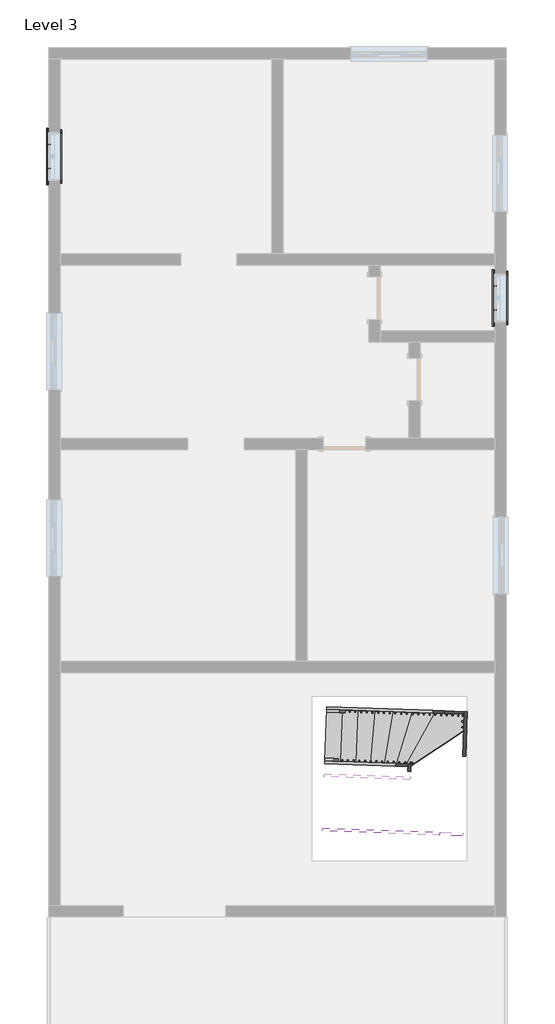
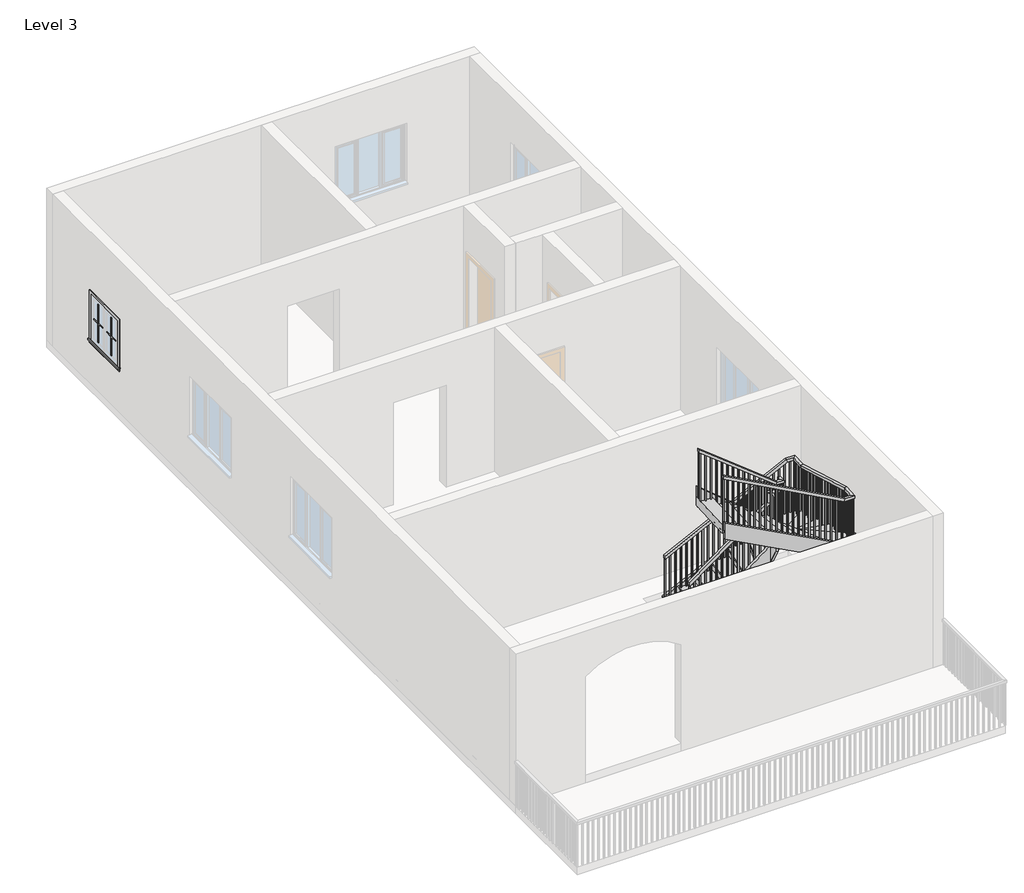
# One storey, part 3 of 3: 8 members, 8 proxies, 2 railings, 1 stair flight.
"""IFC4 building model written with IfcOpenShell, lengths in millimetres."""

from ifc_helpers import new_model, si_unit, frame, origin, place, context, project, spatial, polyline, outline, extrude, faceted_brep, transform, mapped, element, save
from components import muntin_pattern_2x2_muntin_pattern_2x2_b3fe6957, muntin_pattern_2x2_muntin_pattern_2x2_3e0ecaf2, trim_window_exterior_flat_with_sill_41619996, trim_window_interior_flat_picture_frame_51c85655, stair_flight_664b5221

model = new_model("IFC4")

# Units and contexts
model_context = context("Model", 3, world=origin())
ifc_project = project(units=[si_unit("LENGTHUNIT", "METRE", prefix="MILLI")], contexts=[model_context])

# Site, building, storey
site = spatial("IfcSite", under=ifc_project)
building = spatial("IfcBuilding", under=site)
storey = spatial("IfcBuildingStorey", under=building, Name="Level 3", Elevation=6096.0)

# Proxies
placement = place(None, origin())
muntin_pattern_2x2_muntin_pattern_2x2_shape = muntin_pattern_2x2_muntin_pattern_2x2_b3fe6957(model_context)
element("IfcBuildingElementProxy", 1, Name="Muntin Pattern_2x2 : Muntin Pattern_2x2", ObjectType="Muntin Pattern_2x2 : Muntin Pattern_2x2", at=placement, inside=storey, context=model_context, shape_type="MappedRepresentation", body=[
    mapped(muntin_pattern_2x2_muntin_pattern_2x2_shape, transform((-14939.9876504, 9248.016357, 7080.25), x_axis=(0.0, 1.0, 0.0), y_axis=(-1.0, 0.0, 0.0), z_axis=(0.0, 0.0, 1.0))),
])
element("IfcBuildingElementProxy", 2, Name="Muntin Pattern_2x2 : Muntin Pattern_2x2", ObjectType="Muntin Pattern_2x2 : Muntin Pattern_2x2", at=placement, inside=storey, context=model_context, shape_type="MappedRepresentation", body=[
    mapped(muntin_pattern_2x2_muntin_pattern_2x2_shape, transform((-7015.1876504, 6733.416357, 7080.25), x_axis=(0.0, 1.0, 0.0), y_axis=(-1.0, 0.0, 0.0), z_axis=(0.0, 0.0, 1.0))),
])
muntin_pattern_2x2_muntin_pattern_2x2_2_shape = muntin_pattern_2x2_muntin_pattern_2x2_3e0ecaf2(model_context)
element("IfcBuildingElementProxy", 3, Name="Muntin Pattern_2x2 : Muntin Pattern_2x2", ObjectType="Muntin Pattern_2x2 : Muntin Pattern_2x2", at=placement, inside=storey, context=model_context, shape_type="MappedRepresentation", body=[
    mapped(muntin_pattern_2x2_muntin_pattern_2x2_2_shape, transform((-14939.9876504, 9676.641357, 7080.25), x_axis=(0.0, -1.0, 0.0), y_axis=(1.0, 0.0, 0.0), z_axis=(0.0, 0.0, 1.0))),
])
element("IfcBuildingElementProxy", 4, Name="Muntin Pattern_2x2 : Muntin Pattern_2x2", ObjectType="Muntin Pattern_2x2 : Muntin Pattern_2x2", at=placement, inside=storey, context=model_context, shape_type="MappedRepresentation", body=[
    mapped(muntin_pattern_2x2_muntin_pattern_2x2_2_shape, transform((-7015.1876504, 7162.041357, 7080.25), x_axis=(0.0, -1.0, 0.0), y_axis=(1.0, 0.0, 0.0), z_axis=(0.0, 0.0, 1.0))),
])
trim_window_exterior_flat_with_sill_shape = trim_window_exterior_flat_with_sill_41619996(model_context)
element("IfcBuildingElementProxy", 5, Name="Trim-Window-Exterior-Flat : with Sill", ObjectType="Trim-Window-Exterior-Flat : with Sill", at=placement, inside=storey, context=model_context, shape_type="MappedRepresentation", body=[
    mapped(trim_window_exterior_flat_with_sill_shape, transform((-14949.5126504, 9462.328857, 7924.8), x_axis=(0.0, -1.0, 0.0), y_axis=(0.0, 0.0, 1.0), z_axis=(-1.0, 0.0, 0.0))),
])
element("IfcBuildingElementProxy", 6, Name="Trim-Window-Exterior-Flat : with Sill", ObjectType="Trim-Window-Exterior-Flat : with Sill", at=placement, inside=storey, context=model_context, shape_type="MappedRepresentation", body=[
    mapped(trim_window_exterior_flat_with_sill_shape, transform((-7024.7126504, 6947.728857, 7924.8), x_axis=(0.0, -1.0, 0.0), y_axis=(0.0, 0.0, 1.0), z_axis=(-1.0, 0.0, 0.0))),
])
trim_window_interior_flat_picture_frame_shape = trim_window_interior_flat_picture_frame_51c85655(model_context)
element("IfcBuildingElementProxy", 7, Name="Trim-Window-Interior-Flat : Picture Frame", ObjectType="Trim-Window-Interior-Flat : Picture Frame", at=placement, inside=storey, context=model_context, shape_type="MappedRepresentation", body=[
    mapped(trim_window_interior_flat_picture_frame_shape, transform((-14746.3126504, 9462.328857, 7924.8), x_axis=(0.0, 1.0, 0.0), y_axis=(0.0, 0.0, 1.0), z_axis=(1.0, 0.0, 0.0))),
])
element("IfcBuildingElementProxy", 8, Name="Trim-Window-Interior-Flat : Picture Frame", ObjectType="Trim-Window-Interior-Flat : Picture Frame", at=placement, inside=storey, context=model_context, shape_type="MappedRepresentation", body=[
    mapped(trim_window_interior_flat_picture_frame_shape, transform((-6821.5126504, 6947.728857, 7924.8), x_axis=(0.0, 1.0, 0.0), y_axis=(0.0, 0.0, 1.0), z_axis=(1.0, 0.0, 0.0))),
])

# Members
element("IfcMember", 9, ObjectType="Stringer - 2\" Width", at=placement, inside=storey, context=model_context, shape_type="SweptSolid", body=[
    extrude(outline(polyline([(157.0794453, -304.8), (51.8818925, -100.6726296), (247.2290139, 0.0), (2348.3102094, 0.0), (2505.3896547, -304.8), (157.0794453, -304.8)])), frame((-10006.394185, -363.3128759, 5982.7449378), z_axis=(0.03595828761805288, 0.9993532916599501, 0.0), x_axis=(0.8883269481492082, -0.03196338688929392, 0.4580977789626134)), (0.0, 0.0, 1.0), 50.8),
])
element("IfcMember", 10, ObjectType="Stringer - 2\" Width", at=placement, inside=storey, context=model_context, shape_type="SweptSolid", body=[
    extrude(outline(polyline([(-7920.3269434, -438.3728236), (-7918.5002624, -387.6056764), (-7564.0151591, -400.3606025), (-7565.8418401, -451.1277497), (-7920.3269434, -438.3728236)])), frame((0.0, 0.0, 7058.500629), z_axis=(0.0, 0.0, 1.0), x_axis=(1.0, 0.0, 0.0)), (0.0, 0.0, 1.0), 342.8950162),
])
element("IfcMember", 11, ObjectType="Stringer - 2\" Width", at=placement, inside=storey, context=model_context, shape_type="SweptSolid", body=[
    extrude(outline(polyline([(-141.4966894, -274.7041443), (-53.351137, 0.0), (2175.2349578, 0.0), (2210.4467651, -11.2985708), (2109.3071449, -326.4985112), (19.9195916, -326.4985112), (-141.4966894, -274.7041443)])), frame((-7515.0746928, -452.9544307, 7401.3956453), z_axis=(-0.9993532916599502, 0.035958287618053086, 0.0), x_axis=(-0.034238839346999, -0.9515663584286188, 0.30553095978487654)), (0.0, 0.0, 1.0), 50.8),
])
element("IfcMember", 12, ObjectType="Stringer - 2\" Width", at=placement, inside=storey, context=model_context, shape_type="SweptSolid", body=[
    extrude(outline(polyline([(-7590.8819548, -2559.7910402), (-7592.7086358, -2610.5581874), (-7997.9608864, -2595.9765803), (-7996.1342054, -2545.2094331), (-7590.8819548, -2559.7910402)])), frame((0.0, 0.0, 7745.8904473), z_axis=(0.0, 0.0, 1.0), x_axis=(1.0, 0.0, 0.0)), (0.0, 0.0, 1.0), 320.1068224),
])
element("IfcMember", 13, ObjectType="Stringer - 2\" Width", at=placement, inside=storey, context=model_context, shape_type="SweptSolid", body=[
    extrude(outline(polyline([(-146.6402244, -284.5435333), (0.0, 0.0), (2348.3102094, 0.0), (2201.669985, -284.5435333), (-146.6402244, -284.5435333)])), frame((-7997.9608864, -2595.9765803, 8065.9972697), z_axis=(0.03595828761805283, 0.9993532916599502, 0.0), x_axis=(-0.8883269481492087, 0.03196338688929389, 0.45809777896261245)), (0.0, 0.0, 1.0), 50.8),
])
element("IfcMember", 14, ObjectType="Stringer - 2\" Width", at=placement, inside=storey, context=model_context, shape_type="SweptSolid", body=[
    extrude(outline(polyline([(248.5240347, -304.8), (137.1927864, -168.2588219), (343.5522597, 0.0), (1905.6564494, 0.0), (2154.1804842, -304.8), (248.5240347, -304.8)])), frame((-10041.1011242, -1327.888673, 5878.8988904), z_axis=(0.03595828761805293, 0.9993532916599501, 0.0), x_axis=(0.7745239433168307, -0.02786857756239004, 0.6319303787709498)), (0.0, 0.0, 1.0), 50.8),
])
element("IfcMember", 15, ObjectType="Stringer - 2\" Width", at=placement, inside=storey, context=model_context, shape_type="SweptSolid", body=[
    extrude(outline(polyline([(-470.0446027, -275.2513009), (0.0, 0.0), (408.9230004, 1e-07), (420.0212921, -18.9524702), (-68.1184117, -304.7999999), (-452.7413132, -304.8), (-470.0446027, -275.2513009)])), frame((-8512.5307482, -1332.0561414, 7669.2682978), z_axis=(-0.9993532916599502, 0.035958287618050686, 0.0), x_axis=(-0.0181704548133234, -0.5049935642524214, 0.8629318250218337)), (0.0, 0.0, 1.0), 50.8),
])
element("IfcMember", 16, ObjectType="Stringer - 2\" Width", at=placement, inside=storey, context=model_context, shape_type="SweptSolid", body=[
    extrude(outline(polyline([(-248.5240348, -304.8), (0.0, 0.0), (1971.2027087, 0.0), (1722.6786739, -304.8), (-248.5240348, -304.8)])), frame((-8522.5774937, -1611.2754511, 8022.1409689), z_axis=(0.03595828761805281, 0.9993532916599503, 0.0), x_axis=(-0.7745239433168302, 0.027868577562389925, 0.6319303787709504)), (0.0, 0.0, 1.0), 50.8),
])

# Railings
element("IfcRailing", 17, ObjectType="Handrail - Rectangular", at=placement, inside=storey, context=model_context, shape_type="SolidModel", body=[
    faceted_brep([(-10037.4477622, -1226.3543786, 7179.7333333), (-10037.4477622, -1226.3543786, 7115.4000346), (-10039.2744432, -1277.1215258, 7115.4000346), (-10039.2744432, -1277.1215258, 7179.7333333), (-8586.854788, -1278.5489726, 8307.6191036), (-8536.0876408, -1280.3756536, 8282.7590024), (-8537.9143218, -1331.1428009, 8282.7590024), (-8588.681469, -1329.3161198, 8307.6191036), (-8586.854788, -1278.5489726, 8510.6281882), (-8536.0876408, -1280.3756536, 8459.8281882), (-8537.9143218, -1331.1428009, 8459.8281882), (-8588.681469, -1329.3161198, 8510.6281882), (-8459.9369199, -1283.1156752, 8510.6281882), (-8459.9369199, -1283.1156752, 8459.8281882), (-8512.5307482, -1332.0561414, 8459.8281882), (-8512.5307482, -1332.0561414, 8510.6281882), (-8464.5036225, -1410.0335432, 8510.6281882), (-8465.5507758, -1439.136044, 8459.8281882), (-8516.317923, -1437.309363, 8459.8281882), (-8515.2707697, -1408.2068622, 8510.6281882), (-8469.070325, -1536.9514112, 8727.5051451), (-8470.897006, -1587.7185585, 8713.7256424), (-8521.6641532, -1585.8918774, 8713.7256424), (-8519.8374722, -1535.1247302, 8727.5051451), (-8469.070325, -1536.9514112, 8930.5142297), (-8470.897006, -1587.7185585, 8879.7142297), (-8521.6641532, -1585.8918774, 8879.7142297), (-8519.8374722, -1535.1247302, 8930.5142297), (-8473.6370275, -1663.8692793, 8930.5142297), (-8473.6370275, -1663.8692793, 8879.7142297), (-8522.5774937, -1611.2754511, 8879.7142297), (-8522.5774937, -1611.2754511, 8930.5142297), (-8600.5548956, -1659.3025768, 8930.5142297), (-8617.9603, -1658.6763032, 8879.7142297), (-8616.133619, -1607.909156, 8879.7142297), (-8598.7282145, -1608.5354295, 8930.5142297), (-10051.1478698, -1607.1079827, 10058.4), (-10049.3211887, -1556.3408355, 10058.4), (-10049.3211887, -1556.3408355, 9994.0667013), (-10051.1478698, -1607.1079827, 9994.0667013)], [[[0, 1, 2, 3]], [[1, 0, 4, 5]], [[2, 1, 5, 6]], [[3, 2, 6, 7]], [[0, 3, 7, 4]], [[5, 4, 8, 9]], [[6, 5, 9, 10]], [[7, 6, 10, 11]], [[4, 7, 11, 8]], [[9, 8, 12, 13]], [[10, 9, 13, 14]], [[11, 10, 14, 15]], [[8, 11, 15, 12]], [[13, 12, 16, 17]], [[14, 13, 17, 18]], [[15, 14, 18, 19]], [[12, 15, 19, 16]], [[17, 16, 20, 21]], [[18, 17, 21, 22]], [[19, 18, 22, 23]], [[16, 19, 23, 20]], [[21, 20, 24, 25]], [[22, 21, 25, 26]], [[23, 22, 26, 27]], [[20, 23, 27, 24]], [[25, 24, 28, 29]], [[26, 25, 29, 30]], [[27, 26, 30, 31]], [[24, 27, 31, 28]], [[29, 28, 32, 33]], [[30, 29, 33, 34]], [[31, 30, 34, 35]], [[28, 31, 35, 32]], [[36, 37, 38, 39]], [[33, 32, 36, 39]], [[34, 33, 39, 38]], [[35, 34, 38, 37]], [[32, 35, 37, 36]]]),
    extrude(outline(polyline([(236.0012245, -19.05), (221.1987754, 0.0), (1225.3637939, 0.0), (1225.3637939, -19.05), (236.0012245, -19.05)])), frame((-10030.9830199, -1591.9482723, 10200.0304606), z_axis=(0.0359582876180528, 0.9993532916599503, 0.0), x_axis=(0.0, 0.0, -1.0)), (0.0, 0.0, 1.0), 19.05),
    extrude(outline(polyline([(236.0012246, -19.05), (221.1987755, 0.0), (1146.417399, 0.0), (1146.417399, -19.05), (236.0012246, -19.05)])), frame((-9929.4487255, -1595.6016343, 10121.0840657), z_axis=(0.0359582876180528, 0.9993532916599503, 0.0), x_axis=(0.0, 0.0, -1.0)), (0.0, 0.0, 1.0), 19.05),
    extrude(outline(polyline([(236.0012245, -19.05), (221.1987755, 0.0), (1067.471004, 0.0), (1067.471004, -19.05), (236.0012245, -19.05)])), frame((-9827.914431, -1599.2549963, 10042.1376707), z_axis=(0.0359582876180528, 0.9993532916599503, 0.0), x_axis=(0.0, 0.0, -1.0)), (0.0, 0.0, 1.0), 19.05),
    extrude(outline(polyline([(236.0012245, -19.05), (221.1987754, 0.0), (1157.8579424, 0.0), (1157.8579424, -19.05), (236.0012245, -19.05)])), frame((-9726.3801366, -1602.9083583, 9963.1912757), z_axis=(0.0359582876180528, 0.9993532916599503, 0.0), x_axis=(0.0, 0.0, -1.0)), (0.0, 0.0, 1.0), 19.05),
    extrude(outline(polyline([(236.0012246, -19.05), (221.1987755, 0.0), (1078.9115475, 0.0), (1078.9115475, -19.05), (236.0012246, -19.05)])), frame((-9624.8458422, -1606.5617203, 9884.2448808), z_axis=(0.0359582876180528, 0.9993532916599503, 0.0), x_axis=(0.0, 0.0, -1.0)), (0.0, 0.0, 1.0), 19.05),
    extrude(outline(polyline([(236.0012245, -19.05), (221.1987755, 0.0), (999.9651525, 0.0), (999.9651525, -19.05), (236.0012245, -19.05)])), frame((-9523.3115477, -1610.2150824, 9805.2984858), z_axis=(0.0359582876180528, 0.9993532916599503, 0.0), x_axis=(0.0, 0.0, -1.0)), (0.0, 0.0, 1.0), 19.05),
    extrude(outline(polyline([(236.0012245, -19.05), (221.1987754, 0.0), (1090.3520908, 0.0), (1090.3520908, -19.05), (236.0012245, -19.05)])), frame((-9421.7772533, -1613.8684444, 9726.3520908), z_axis=(0.0359582876180528, 0.9993532916599503, 0.0), x_axis=(0.0, 0.0, -1.0)), (0.0, 0.0, 1.0), 19.05),
    extrude(outline(polyline([(236.0012246, -19.05), (221.1987755, 0.0), (1011.4056959, 0.0), (1011.4056959, -19.05), (236.0012246, -19.05)])), frame((-9320.2429589, -1617.5218064, 9647.4056959), z_axis=(0.0359582876180528, 0.9993532916599503, 0.0), x_axis=(0.0, 0.0, -1.0)), (0.0, 0.0, 1.0), 19.05),
    extrude(outline(polyline([(236.0012245, -19.05), (221.1987755, 0.0), (1101.7926342, 0.0), (1101.7926342, -19.05), (236.0012245, -19.05)])), frame((-9218.7086644, -1621.1751684, 9568.4593009), z_axis=(0.0359582876180528, 0.9993532916599503, 0.0), x_axis=(0.0, 0.0, -1.0)), (0.0, 0.0, 1.0), 19.05),
    extrude(outline(polyline([(236.0012245, -19.05), (221.1987755, 0.0), (1022.8462392, 0.0), (1022.8462392, -19.05), (236.0012245, -19.05)])), frame((-9117.17437, -1624.8285304, 9489.5129059), z_axis=(0.0359582876180528, 0.9993532916599503, 0.0), x_axis=(0.0, 0.0, -1.0)), (0.0, 0.0, 1.0), 19.05),
    extrude(outline(polyline([(236.0012245, -19.05), (221.1987754, 0.0), (943.8998442, 0.0), (943.8998442, -19.05), (236.0012245, -19.05)])), frame((-9015.6400756, -1628.4818925, 9410.5665109), z_axis=(0.0359582876180528, 0.9993532916599503, 0.0), x_axis=(0.0, 0.0, -1.0)), (0.0, 0.0, 1.0), 19.05),
    extrude(outline(polyline([(236.0012246, -19.05), (221.1987755, 0.0), (1034.2867827, 0.0), (1034.2867827, -19.05), (236.0012246, -19.05)])), frame((-8914.1057811, -1632.1352545, 9331.620116), z_axis=(0.0359582876180528, 0.9993532916599503, 0.0), x_axis=(0.0, 0.0, -1.0)), (0.0, 0.0, 1.0), 19.05),
    extrude(outline(polyline([(236.0012245, -19.05), (221.1987755, 0.0), (955.3403877, 0.0), (955.3403877, -19.05), (236.0012245, -19.05)])), frame((-8812.5714867, -1635.7886165, 9252.673721), z_axis=(0.0359582876180528, 0.9993532916599503, 0.0), x_axis=(0.0, 0.0, -1.0)), (0.0, 0.0, 1.0), 19.05),
    extrude(outline(polyline([(236.0012245, -19.05), (221.1987754, 0.0), (1045.727326, 0.0), (1045.727326, -19.05), (236.0012245, -19.05)])), frame((-8711.0371923, -1639.4419785, 9173.727326), z_axis=(0.0359582876180528, 0.9993532916599503, 0.0), x_axis=(0.0, 0.0, -1.0)), (0.0, 0.0, 1.0), 19.05),
    extrude(outline(polyline([(236.0012246, -19.05), (221.1987755, 0.0), (966.7809311, 0.0), (966.7809311, -19.05), (236.0012246, -19.05)])), frame((-8609.5028978, -1643.0953406, 9094.7809311), z_axis=(0.0359582876180528, 0.9993532916599503, 0.0), x_axis=(0.0, 0.0, -1.0)), (0.0, 0.0, 1.0), 19.05),
    extrude(outline(polyline([(-8506.3702575, -1602.3274488), (-8487.3325773, -1603.0124541), (-8488.0175827, -1622.0501344), (-8507.0552629, -1621.365129), (-8506.3702575, -1602.3274488)])), frame((0.0, 0.0, 7789.3333333), z_axis=(0.0, 0.0, 1.0), x_axis=(1.0, 0.0, 0.0)), (0.0, 0.0, 1.0), 1090.3808964),
    extrude(outline(polyline([(244.8657718, -19.05), (212.3342282, 0.0), (1192.1994682, 0.0), (1192.1994682, -19.05), (244.8657718, -19.05)])), frame((-8484.3642207, -1520.5158399, 8812.1994682), z_axis=(-0.9993532916599502, 0.035958287618050686, 0.0), x_axis=(0.0, 0.0, -1.0)), (0.0, 0.0, 1.0), 19.05),
    extrude(outline(polyline([(244.8657717, -19.05), (212.3342282, 0.0), (1188.0312359, 0.0), (1188.0312359, -19.05), (244.8657717, -19.05)])), frame((-8480.7108586, -1418.9815455, 8638.6979026), z_axis=(-0.9993532916599502, 0.035958287618050686, 0.0), x_axis=(0.0, 0.0, -1.0)), (0.0, 0.0, 1.0), 19.05),
    extrude(outline(polyline([(-8525.208029, -1315.7147199), (-8524.5230236, -1296.6770397), (-8505.4853434, -1297.3620451), (-8506.1703488, -1316.3997253), (-8525.208029, -1315.7147199)])), frame((0.0, 0.0, 7281.3333333), z_axis=(0.0, 0.0, 1.0), x_axis=(1.0, 0.0, 0.0)), (0.0, 0.0, 1.0), 1178.4948549),
    extrude(outline(polyline([(221.1987754, -19.05), (236.0012245, 0.0), (1337.2495642, 0.0), (1337.2495642, -19.05), (221.1987754, -19.05)])), frame((-8626.7423234, -1312.0613579, 8449.2495642), z_axis=(0.035958287618052934, 0.9993532916599503, 0.0), x_axis=(0.0, 0.0, -1.0)), (0.0, 0.0, 1.0), 19.05),
    extrude(outline(polyline([(221.1987755, -19.0500001), (236.0012246, 0.0), (1258.3031693, 0.0), (1258.3031693, -19.0500001), (221.1987755, -19.0500001)])), frame((-8728.2766179, -1308.4079959, 8370.3031693), z_axis=(0.035958287618052934, 0.9993532916599503, 0.0), x_axis=(0.0, 0.0, -1.0)), (0.0, 0.0, 1.0), 19.05),
    extrude(outline(polyline([(221.1987755, -19.05), (236.0012245, 0.0), (1348.6901076, 0.0), (1348.6901076, -19.05), (221.1987755, -19.05)])), frame((-8829.8109123, -1304.7546339, 8291.3567743), z_axis=(0.035958287618052934, 0.9993532916599503, 0.0), x_axis=(0.0, 0.0, -1.0)), (0.0, 0.0, 1.0), 19.05),
    extrude(outline(polyline([(221.1987754, -19.05), (236.0012245, 0.0), (1269.7437126, 0.0), (1269.7437126, -19.05), (221.1987754, -19.05)])), frame((-8931.3452067, -1301.1012718, 8212.4103793), z_axis=(0.035958287618052934, 0.9993532916599503, 0.0), x_axis=(0.0, 0.0, -1.0)), (0.0, 0.0, 1.0), 19.05),
    extrude(outline(polyline([(221.1987755, -19.05), (236.0012246, 0.0), (1360.1306511, 0.0), (1360.1306511, -19.05), (221.1987755, -19.05)])), frame((-9032.8795011, -1297.4479098, 8133.4639844), z_axis=(0.035958287618052934, 0.9993532916599503, 0.0), x_axis=(0.0, 0.0, -1.0)), (0.0, 0.0, 1.0), 19.05),
    extrude(outline(polyline([(221.1987755, -19.05), (236.0012245, 0.0), (1281.1842561, 0.0), (1281.1842561, -19.05), (221.1987755, -19.05)])), frame((-9134.4137956, -1293.7945478, 8054.5175894), z_axis=(0.035958287618052934, 0.9993532916599503, 0.0), x_axis=(0.0, 0.0, -1.0)), (0.0, 0.0, 1.0), 19.05),
    extrude(outline(polyline([(221.1987755, -19.05), (236.0012245, 0.0), (1371.5711944, 0.0), (1371.5711944, -19.05), (221.1987755, -19.05)])), frame((-9235.94809, -1290.1411858, 7975.5711944), z_axis=(0.035958287618052934, 0.9993532916599503, 0.0), x_axis=(0.0, 0.0, -1.0)), (0.0, 0.0, 1.0), 19.05),
    extrude(outline(polyline([(221.1987754, -19.05), (236.0012245, 0.0), (1292.6247994, 0.0), (1292.6247994, -19.05), (221.1987754, -19.05)])), frame((-9337.4823844, -1286.4878237, 7896.6247994), z_axis=(0.035958287618052934, 0.9993532916599503, 0.0), x_axis=(0.0, 0.0, -1.0)), (0.0, 0.0, 1.0), 19.05),
    extrude(outline(polyline([(221.1987755, -19.05), (236.0012246, 0.0), (1213.6784045, 0.0), (1213.6784045, -19.05), (221.1987755, -19.05)])), frame((-9439.0166789, -1282.8344617, 7817.6784045), z_axis=(0.035958287618052934, 0.9993532916599503, 0.0), x_axis=(0.0, 0.0, -1.0)), (0.0, 0.0, 1.0), 19.05),
    extrude(outline(polyline([(221.1987755, -19.05), (236.0012245, 0.0), (1304.0653428, 0.0), (1304.0653428, -19.05), (221.1987755, -19.05)])), frame((-9540.5509733, -1279.1810997, 7738.7320095), z_axis=(0.035958287618052934, 0.9993532916599503, 0.0), x_axis=(0.0, 0.0, -1.0)), (0.0, 0.0, 1.0), 19.05),
    extrude(outline(polyline([(221.1987754, -19.05), (236.0012245, 0.0), (1225.1189478, 0.0), (1225.1189478, -19.05), (221.1987754, -19.05)])), frame((-9642.0852677, -1275.5277377, 7659.7856145), z_axis=(0.035958287618052934, 0.9993532916599503, 0.0), x_axis=(0.0, 0.0, -1.0)), (0.0, 0.0, 1.0), 19.05),
    extrude(outline(polyline([(221.1987755, -19.05), (236.0012246, 0.0), (1146.1725529, 0.0), (1146.1725529, -19.05), (221.1987755, -19.05)])), frame((-9743.6195622, -1271.8743757, 7580.8392196), z_axis=(0.035958287618052934, 0.9993532916599503, 0.0), x_axis=(0.0, 0.0, -1.0)), (0.0, 0.0, 1.0), 19.05),
    extrude(outline(polyline([(221.1987755, -19.05), (236.0012245, 0.0), (1236.5594913, 0.0), (1236.5594913, -19.05), (221.1987755, -19.05)])), frame((-9845.1538566, -1268.2210136, 7501.8928246), z_axis=(0.035958287618052934, 0.9993532916599503, 0.0), x_axis=(0.0, 0.0, -1.0)), (0.0, 0.0, 1.0), 19.05),
    extrude(outline(polyline([(221.1987755, -19.05), (236.0012245, 0.0), (1157.6130963, 0.0), (1157.6130963, -19.05), (221.1987755, -19.05)])), frame((-9946.688151, -1264.5676516, 7422.9464296), z_axis=(0.035958287618052934, 0.9993532916599503, 0.0), x_axis=(0.0, 0.0, -1.0)), (0.0, 0.0, 1.0), 19.05),
    extrude(outline(polyline([(-8507.283598, -1627.7110224), (-8488.2459178, -1628.3960278), (-8488.9309232, -1647.433708), (-8507.9686034, -1646.7487026), (-8507.283598, -1627.7110224)])), frame((0.0, 0.0, 7958.6666667), z_axis=(0.0, 0.0, 1.0), x_axis=(1.0, 0.0, 0.0)), (0.0, 0.0, 1.0), 921.0475631),
    extrude(outline(polyline([(-8496.0951768, -1316.7622457), (-8495.4101715, -1297.7245655), (-8476.3724912, -1298.4095708), (-8477.0574966, -1317.4472511), (-8496.0951768, -1316.7622457)])), frame((0.0, 0.0, 7281.3333333), z_axis=(0.0, 0.0, 1.0), x_axis=(1.0, 0.0, 0.0)), (0.0, 0.0, 1.0), 1178.4948549),
    extrude(outline(polyline([(236.0012245, -19.05), (221.1987755, 0.0), (1240.5988101, 0.0), (1240.5988101, -19.05), (236.0012245, -19.05)])), frame((-10050.5770319, -1591.2432492, 10215.2654768), z_axis=(0.0359582876180528, 0.9993532916599503, 0.0), x_axis=(0.0, 0.0, -1.0)), (0.0, 0.0, 1.0), 19.05),
    extrude(outline(polyline([(221.1987755, -19.05), (236.0012246, 0.0), (1086.0679259, 0.0), (1086.0679259, -19.05), (221.1987755, -19.05)])), frame((-10038.7036054, -1261.2567923, 7351.4012592), z_axis=(0.035958287618052934, 0.9993532916599503, 0.0), x_axis=(0.0, 0.0, -1.0)), (0.0, 0.0, 1.0), 19.05),
])
element("IfcRailing", 18, ObjectType="Handrail - Rectangular", at=placement, inside=storey, context=model_context, shape_type="SolidModel", body=[
    faceted_brep([(-10006.394185, -363.3128759, 7179.7333333), (-10006.394185, -363.3128759, 7122.2742652), (-10008.220866, -414.0800231, 7122.2742652), (-10008.220866, -414.0800231, 7179.7333333), (-7750.1292126, -444.496803, 8373.0239201), (-7737.5382959, -444.9498438, 8322.2239201), (-7739.364977, -495.716991, 8322.2239201), (-7751.9558936, -495.2639503, 8373.0239201), (-7565.8418401, -451.1277497, 8373.0239201), (-7565.8418401, -451.1277497, 8322.2239201), (-7618.4356683, -500.0682159, 8322.2239201), (-7618.4356683, -500.0682159, 8373.0239201), (-7576.1730834, -738.2538248, 8373.0239201), (-7576.4589725, -746.1992592, 8322.2239201), (-7627.2261197, -744.3725782, 8322.2239201), (-7626.9402306, -736.4271438, 8373.0239201), (-7631.3178587, -2270.838284, 8865.1094132), (-7631.6037478, -2278.7837184, 8814.3094132), (-7682.370895, -2276.9570374, 8814.3094132), (-7682.0850059, -2269.011603, 8865.1094132), (-7641.649102, -2557.9643591, 8865.1094132), (-7641.649102, -2557.9643591, 8814.3094132), (-7690.5895682, -2505.3705309, 8814.3094132), (-7690.5895682, -2505.3705309, 8865.1094132), (-7825.9364745, -2551.3334125, 8865.1094132), (-7838.5273911, -2550.8803717, 8814.3094132), (-7836.7007101, -2500.1132245, 8814.3094132), (-7824.1097935, -2500.5662653, 8865.1094132), (-10082.2014469, -2470.1494854, 10058.4), (-10080.3747659, -2419.3823382, 10058.4), (-10080.3747659, -2419.3823382, 10000.9409318), (-10082.2014469, -2470.1494854, 10000.9409318)], [[[0, 1, 2, 3]], [[1, 0, 4, 5]], [[2, 1, 5, 6]], [[3, 2, 6, 7]], [[0, 3, 7, 4]], [[5, 4, 8, 9]], [[6, 5, 9, 10]], [[7, 6, 10, 11]], [[4, 7, 11, 8]], [[9, 8, 12, 13]], [[10, 9, 13, 14]], [[11, 10, 14, 15]], [[8, 11, 15, 12]], [[13, 12, 16, 17]], [[14, 13, 17, 18]], [[15, 14, 18, 19]], [[12, 15, 19, 16]], [[17, 16, 20, 21]], [[18, 17, 21, 22]], [[19, 18, 22, 23]], [[16, 19, 23, 20]], [[21, 20, 24, 25]], [[22, 21, 25, 26]], [[23, 22, 26, 27]], [[20, 23, 27, 24]], [[28, 29, 30, 31]], [[25, 24, 28, 31]], [[26, 25, 31, 30]], [[27, 26, 30, 29]], [[24, 27, 29, 28]]]),
    extrude(outline(polyline([(223.5656878, 19.05), (1212.6274313, 19.05), (1212.6274313, 0.0), (233.6343122, 0.0), (223.5656878, 19.05)])), frame((-9992.2317697, -2457.5014613, 10187.294098), z_axis=(0.035958287618052934, 0.9993532916599503, 0.0), x_axis=(0.0, 0.0, -1.0)), (0.0, 0.0, 1.0), 19.05),
    extrude(outline(polyline([(223.5656878, 19.05), (1158.9281011, 19.05), (1158.9281011, 0.0), (233.6343122, 0.0), (223.5656878, 19.05)])), frame((-9890.6974752, -2461.1548233, 10133.5947678), z_axis=(0.035958287618052934, 0.9993532916599503, 0.0), x_axis=(0.0, 0.0, -1.0)), (0.0, 0.0, 1.0), 19.05),
    extrude(outline(polyline([(223.5656878, 19.05), (1274.5621043, 19.05), (1274.5621043, 0.0), (233.6343122, 0.0), (223.5656878, 19.05)])), frame((-9789.1631808, -2464.8081854, 10079.8954376), z_axis=(0.035958287618052934, 0.9993532916599503, 0.0), x_axis=(0.0, 0.0, -1.0)), (0.0, 0.0, 1.0), 19.05),
    extrude(outline(polyline([(223.5656878, 19.05), (1220.8627741, 19.05), (1220.8627741, 0.0), (233.6343122, 0.0), (223.5656878, 19.05)])), frame((-9687.6288864, -2468.4615474, 10026.1961074), z_axis=(0.035958287618052934, 0.9993532916599503, 0.0), x_axis=(0.0, 0.0, -1.0)), (0.0, 0.0, 1.0), 19.05),
    extrude(outline(polyline([(223.5656878, 19.05), (1167.1634439, 19.05), (1167.1634439, 0.0), (233.6343122, 0.0), (223.5656878, 19.05)])), frame((-9586.0945919, -2472.1149094, 9972.4967772), z_axis=(0.035958287618052934, 0.9993532916599503, 0.0), x_axis=(0.0, 0.0, -1.0)), (0.0, 0.0, 1.0), 19.05),
    extrude(outline(polyline([(223.5656878, 19.05), (1282.797447, 19.05), (1282.797447, 0.0), (233.6343122, 0.0), (223.5656878, 19.05)])), frame((-9484.5602975, -2475.7682714, 9918.797447), z_axis=(0.035958287618052934, 0.9993532916599503, 0.0), x_axis=(0.0, 0.0, -1.0)), (0.0, 0.0, 1.0), 19.05),
    extrude(outline(polyline([(223.5656878, 19.05), (1229.0981168, 19.05), (1229.0981168, 0.0), (233.6343122, 0.0), (223.5656878, 19.05)])), frame((-9383.0260031, -2479.4216334, 9865.0981168), z_axis=(0.035958287618052934, 0.9993532916599503, 0.0), x_axis=(0.0, 0.0, -1.0)), (0.0, 0.0, 1.0), 19.05),
    extrude(outline(polyline([(223.5656878, 19.05), (1175.3987866, 19.05), (1175.3987866, 0.0), (233.6343122, 0.0), (223.5656878, 19.05)])), frame((-9281.4917086, -2483.0749955, 9811.3987866), z_axis=(0.035958287618052934, 0.9993532916599503, 0.0), x_axis=(0.0, 0.0, -1.0)), (0.0, 0.0, 1.0), 19.05),
    extrude(outline(polyline([(223.5656878, 19.05), (1291.0327897, 19.05), (1291.0327897, 0.0), (233.6343122, 0.0), (223.5656878, 19.05)])), frame((-9179.9574142, -2486.7283575, 9757.6994564), z_axis=(0.035958287618052934, 0.9993532916599503, 0.0), x_axis=(0.0, 0.0, -1.0)), (0.0, 0.0, 1.0), 19.05),
    extrude(outline(polyline([(223.5656878, 19.05), (1237.3334595, 19.05), (1237.3334595, 0.0), (233.6343122, 0.0), (223.5656878, 19.05)])), frame((-9078.4231198, -2490.3817195, 9704.0001262), z_axis=(0.035958287618052934, 0.9993532916599503, 0.0), x_axis=(0.0, 0.0, -1.0)), (0.0, 0.0, 1.0), 19.05),
    extrude(outline(polyline([(223.5656878, 19.05), (1183.6341293, 19.05), (1183.6341293, 0.0), (233.6343122, 0.0), (223.5656878, 19.05)])), frame((-8976.8888253, -2494.0350815, 9650.300796), z_axis=(0.035958287618052934, 0.9993532916599503, 0.0), x_axis=(0.0, 0.0, -1.0)), (0.0, 0.0, 1.0), 19.05),
    extrude(outline(polyline([(223.5656878, 19.05), (1299.2681325, 19.05), (1299.2681325, 0.0), (233.6343122, 0.0), (223.5656878, 19.05)])), frame((-8875.3545309, -2497.6884436, 9596.6014658), z_axis=(0.035958287618052934, 0.9993532916599503, 0.0), x_axis=(0.0, 0.0, -1.0)), (0.0, 0.0, 1.0), 19.05),
    extrude(outline(polyline([(223.5656878, 19.05), (1245.5688023, 19.05), (1245.5688023, 0.0), (233.6343122, 0.0), (223.5656878, 19.05)])), frame((-8773.8202365, -2501.3418056, 9542.9021356), z_axis=(0.035958287618052934, 0.9993532916599503, 0.0), x_axis=(0.0, 0.0, -1.0)), (0.0, 0.0, 1.0), 19.05),
    extrude(outline(polyline([(223.5656878, 19.05), (1191.8694721, 19.05), (1191.8694721, 0.0), (233.6343122, 0.0), (223.5656878, 19.05)])), frame((-8672.285942, -2504.9951676, 9489.2028054), z_axis=(0.035958287618052934, 0.9993532916599503, 0.0), x_axis=(0.0, 0.0, -1.0)), (0.0, 0.0, 1.0), 19.05),
    extrude(outline(polyline([(223.5656878, 19.05), (1138.1701419, 19.05), (1138.1701419, 0.0), (233.6343122, 0.0), (223.5656878, 19.05)])), frame((-8570.7516476, -2508.6485296, 9435.5034752), z_axis=(0.035958287618052934, 0.9993532916599503, 0.0), x_axis=(0.0, 0.0, -1.0)), (0.0, 0.0, 1.0), 19.05),
    extrude(outline(polyline([(223.5656878, 19.05), (1253.804145, 19.05), (1253.804145, 0.0), (233.6343122, 0.0), (223.5656878, 19.05)])), frame((-8469.2173532, -2512.3018916, 9381.804145), z_axis=(0.035958287618052934, 0.9993532916599503, 0.0), x_axis=(0.0, 0.0, -1.0)), (0.0, 0.0, 1.0), 19.05),
    extrude(outline(polyline([(223.5656878, 19.05), (1200.1048148, 19.05), (1200.1048148, 0.0), (233.6343122, 0.0), (223.5656878, 19.05)])), frame((-8367.6830587, -2515.9552537, 9328.1048148), z_axis=(0.035958287618052934, 0.9993532916599503, 0.0), x_axis=(0.0, 0.0, -1.0)), (0.0, 0.0, 1.0), 19.05),
    extrude(outline(polyline([(223.5656878, 19.05), (1146.4054846, 19.05), (1146.4054846, 0.0), (233.6343122, 0.0), (223.5656878, 19.05)])), frame((-8266.1487643, -2519.6086157, 9274.4054846), z_axis=(0.035958287618052934, 0.9993532916599503, 0.0), x_axis=(0.0, 0.0, -1.0)), (0.0, 0.0, 1.0), 19.05),
    extrude(outline(polyline([(223.5656878, 19.05), (1092.7061544, 19.05), (1092.7061544, 0.0), (233.6343122, 0.0), (223.5656878, 19.05)])), frame((-8164.6144699, -2523.2619777, 9220.7061544), z_axis=(0.035958287618052934, 0.9993532916599503, 0.0), x_axis=(0.0, 0.0, -1.0)), (0.0, 0.0, 1.0), 19.05),
    extrude(outline(polyline([(223.5656878, 19.05), (1208.3401575, 19.05), (1208.3401575, 0.0), (233.6343122, 0.0), (223.5656878, 19.05)])), frame((-8063.0801754, -2526.9153397, 9167.0068242), z_axis=(0.035958287618052934, 0.9993532916599503, 0.0), x_axis=(0.0, 0.0, -1.0)), (0.0, 0.0, 1.0), 19.05),
    extrude(outline(polyline([(223.5656878, 19.05), (1154.6408273, 19.05), (1154.6408273, 0.0), (233.6343122, 0.0), (223.5656878, 19.05)])), frame((-7961.545881, -2530.5687018, 9113.307494), z_axis=(0.035958287618052934, 0.9993532916599503, 0.0), x_axis=(0.0, 0.0, -1.0)), (0.0, 0.0, 1.0), 19.05),
    extrude(outline(polyline([(223.5656878, 19.05), (1100.9414971, 19.05), (1100.9414971, 0.0), (233.6343122, 0.0), (223.5656878, 19.05)])), frame((-7860.0115866, -2534.2220638, 9059.6081638), z_axis=(0.035958287618052934, 0.9993532916599503, 0.0), x_axis=(0.0, 0.0, -1.0)), (0.0, 0.0, 1.0), 19.05),
    extrude(outline(polyline([(-7758.4772921, -2537.8754258), (-7777.5149723, -2537.1904204), (-7776.829967, -2518.1527402), (-7757.7922868, -2518.8377456), (-7758.4772921, -2537.8754258)])), frame((0.0, 0.0, 7958.6666667), z_axis=(0.0, 0.0, 1.0), x_axis=(1.0, 0.0, 0.0)), (0.0, 0.0, 1.0), 855.6427466),
    extrude(outline(polyline([(-7655.3446518, -2497.107534), (-7656.0296572, -2516.1452142), (-7675.0673374, -2515.4602088), (-7674.382332, -2496.4225286), (-7655.3446518, -2497.107534)])), frame((0.0, 0.0, 7958.6666667), z_axis=(0.0, 0.0, 1.0), x_axis=(1.0, 0.0, 0.0)), (0.0, 0.0, 1.0), 855.6427466),
    extrude(outline(polyline([(-7651.6912898, -2395.5732396), (-7652.3762952, -2414.6109198), (-7671.4139754, -2413.9259144), (-7670.72897, -2394.8882342), (-7651.6912898, -2395.5732396)])), frame((0.0, 0.0, 7958.6666667), z_axis=(0.0, 0.0, 1.0), x_axis=(1.0, 0.0, 0.0)), (0.0, 0.0, 1.0), 855.6427466),
    extrude(outline(polyline([(-7648.0379278, -2294.0389451), (-7648.7229332, -2313.0766254), (-7667.7606134, -2312.39162), (-7667.075608, -2293.3539398), (-7648.0379278, -2294.0389451)])), frame((0.0, 0.0, 7958.6666667), z_axis=(0.0, 0.0, 1.0), x_axis=(1.0, 0.0, 0.0)), (0.0, 0.0, 1.0), 855.6427466),
    extrude(outline(polyline([(225.5436705, 19.05), (1229.1130279, 19.05), (1229.1130279, 0.0), (231.6563296, 0.0), (225.5436705, 19.05)])), frame((-7644.3845658, -2192.5046507, 9018.4463612), z_axis=(-0.9993532916599501, 0.03595828761805307, 0.0), x_axis=(0.0, 0.0, -1.0)), (0.0, 0.0, 1.0), 19.05),
    extrude(outline(polyline([(225.5436704, 19.05), (1196.5121796, 19.05), (1196.5121796, 0.0), (231.6563295, 0.0), (225.5436704, 19.05)])), frame((-7640.7312037, -2090.9703563, 8985.8455129), z_axis=(-0.9993532916599501, 0.03595828761805307, 0.0), x_axis=(0.0, 0.0, -1.0)), (0.0, 0.0, 1.0), 19.05),
    extrude(outline(polyline([(225.5436705, 19.0500001), (1163.9113314, 19.0500001), (1163.9113314, 0.0), (231.6563295, 0.0), (225.5436705, 19.0500001)])), frame((-7637.0778417, -1989.4360618, 8953.2446647), z_axis=(-0.9993532916599501, 0.03595828761805307, 0.0), x_axis=(0.0, 0.0, -1.0)), (0.0, 0.0, 1.0), 19.05),
    extrude(outline(polyline([(225.5436705, 19.05), (1131.3104832, 19.05), (1131.3104832, 0.0), (231.6563295, 0.0), (225.5436705, 19.05)])), frame((-7633.4244797, -1887.9017674, 8920.6438165), z_axis=(-0.9993532916599501, 0.03595828761805307, 0.0), x_axis=(0.0, 0.0, -1.0)), (0.0, 0.0, 1.0), 19.05),
    extrude(outline(polyline([(225.5436705, 19.05), (1098.709635, 19.05), (1098.709635, 0.0), (231.6563296, 0.0), (225.5436705, 19.05)])), frame((-7629.7711177, -1786.367473, 8888.0429683), z_axis=(-0.9993532916599501, 0.03595828761805307, 0.0), x_axis=(0.0, 0.0, -1.0)), (0.0, 0.0, 1.0), 19.05),
    extrude(outline(polyline([(225.5436705, 19.0500001), (1235.44212, 19.0500001), (1235.44212, 0.0), (231.6563295, 0.0), (225.5436705, 19.0500001)])), frame((-7626.1177556, -1684.8331785, 8855.44212), z_axis=(-0.9993532916599501, 0.03595828761805307, 0.0), x_axis=(0.0, 0.0, -1.0)), (0.0, 0.0, 1.0), 19.05),
    extrude(outline(polyline([(225.5436705, 19.05), (1202.8412718, 19.05), (1202.8412718, 0.0), (231.6563295, 0.0), (225.5436705, 19.05)])), frame((-7622.4643936, -1583.2988841, 8822.8412718), z_axis=(-0.9993532916599501, 0.03595828761805307, 0.0), x_axis=(0.0, 0.0, -1.0)), (0.0, 0.0, 1.0), 19.05),
    extrude(outline(polyline([(225.5436705, 19.05), (1170.2404236, 19.05), (1170.2404236, 0.0), (231.6563296, 0.0), (225.5436705, 19.05)])), frame((-7618.8110316, -1481.7645897, 8790.2404236), z_axis=(-0.9993532916599501, 0.03595828761805307, 0.0), x_axis=(0.0, 0.0, -1.0)), (0.0, 0.0, 1.0), 19.05),
    extrude(outline(polyline([(225.5436704, 19.05), (1137.6395753, 19.05), (1137.6395753, 0.0), (231.6563295, 0.0), (225.5436704, 19.05)])), frame((-7615.1576696, -1380.2302953, 8757.6395753), z_axis=(-0.9993532916599501, 0.03595828761805307, 0.0), x_axis=(0.0, 0.0, -1.0)), (0.0, 0.0, 1.0), 19.05),
    extrude(outline(polyline([(225.5436705, 19.05), (1105.0387271, 19.05), (1105.0387271, 0.0), (231.6563295, 0.0), (225.5436705, 19.05)])), frame((-7611.5043076, -1278.6960008, 8725.0387271), z_axis=(-0.9993532916599501, 0.03595828761805307, 0.0), x_axis=(0.0, 0.0, -1.0)), (0.0, 0.0, 1.0), 19.05),
    extrude(outline(polyline([(225.5436705, 19.05), (1241.7712122, 19.05), (1241.7712122, 0.0), (231.6563295, 0.0), (225.5436705, 19.05)])), frame((-7607.8509455, -1177.1617064, 8692.4378789), z_axis=(-0.9993532916599501, 0.03595828761805307, 0.0), x_axis=(0.0, 0.0, -1.0)), (0.0, 0.0, 1.0), 19.05),
    extrude(outline(polyline([(225.5436705, 19.05), (1209.170364, 19.05), (1209.170364, 0.0), (231.6563296, 0.0), (225.5436705, 19.05)])), frame((-7604.1975835, -1075.627412, 8659.8370307), z_axis=(-0.9993532916599501, 0.03595828761805307, 0.0), x_axis=(0.0, 0.0, -1.0)), (0.0, 0.0, 1.0), 19.05),
    extrude(outline(polyline([(225.5436704, 19.05), (1176.5695157, 19.05), (1176.5695157, 0.0), (231.6563295, 0.0), (225.5436704, 19.05)])), frame((-7600.5442215, -974.0931175, 8627.2361824), z_axis=(-0.9993532916599501, 0.03595828761805307, 0.0), x_axis=(0.0, 0.0, -1.0)), (0.0, 0.0, 1.0), 19.05),
    extrude(outline(polyline([(225.5436705, 19.05), (1143.9686675, 19.05), (1143.9686675, 0.0), (231.6563295, 0.0), (225.5436705, 19.05)])), frame((-7596.8908595, -872.5588231, 8594.6353342), z_axis=(-0.9993532916599501, 0.03595828761805307, 0.0), x_axis=(0.0, 0.0, -1.0)), (0.0, 0.0, 1.0), 19.05),
    extrude(outline(polyline([(225.5436705, 19.05), (1111.3678193, 19.05), (1111.3678193, 0.0), (231.6563295, 0.0), (225.5436705, 19.05)])), frame((-7593.2374974, -771.0245287, 8562.034486), z_axis=(-0.9993532916599501, 0.03595828761805307, 0.0), x_axis=(0.0, 0.0, -1.0)), (0.0, 0.0, 1.0), 19.05),
    extrude(outline(polyline([(-7589.5841354, -669.4902342), (-7590.2691408, -688.5279144), (-7609.306821, -687.842909), (-7608.6218156, -668.8052288), (-7589.5841354, -669.4902342)])), frame((0.0, 0.0, 7281.3333333), z_axis=(0.0, 0.0, 1.0), x_axis=(1.0, 0.0, 0.0)), (0.0, 0.0, 1.0), 1040.8905868),
    extrude(outline(polyline([(-7585.9307734, -567.9559398), (-7586.6157788, -586.99362), (-7605.653459, -586.3086146), (-7604.9684536, -567.2709344), (-7585.9307734, -567.9559398)])), frame((0.0, 0.0, 7281.3333333), z_axis=(0.0, 0.0, 1.0), x_axis=(1.0, 0.0, 0.0)), (0.0, 0.0, 1.0), 1040.8905868),
    extrude(outline(polyline([(-7681.195091, -462.8624332), (-7662.1574108, -463.5474386), (-7662.8424161, -482.5851188), (-7681.8800963, -481.9001134), (-7681.195091, -462.8624332)])), frame((0.0, 0.0, 7281.3333333), z_axis=(0.0, 0.0, 1.0), x_axis=(1.0, 0.0, 0.0)), (0.0, 0.0, 1.0), 1040.8905868),
    extrude(outline(polyline([(233.6343122, 19.05), (1250.9261963, 19.05), (1250.9261963, 0.0), (223.5656878, 0.0), (233.6343122, 19.05)])), frame((-7764.3767106, -478.9317568, 8532.2595296), z_axis=(0.03595828761805286, 0.9993532916599503, 0.0), x_axis=(0.0, 0.0, -1.0)), (0.0, 0.0, 1.0), 19.05),
    extrude(outline(polyline([(233.6343122, 19.05), (1197.2268661, 19.05), (1197.2268661, 0.0), (223.5656878, 0.0), (233.6343122, 19.05)])), frame((-7865.911005, -475.2783948, 8478.5601994), z_axis=(0.03595828761805286, 0.9993532916599503, 0.0), x_axis=(0.0, 0.0, -1.0)), (0.0, 0.0, 1.0), 19.05),
    extrude(outline(polyline([(233.6343122, 19.05), (1143.5275359, 19.05), (1143.5275359, 0.0), (223.5656878, 0.0), (233.6343122, 19.05)])), frame((-7967.4452994, -471.6250327, 8424.8608692), z_axis=(0.03595828761805286, 0.9993532916599503, 0.0), x_axis=(0.0, 0.0, -1.0)), (0.0, 0.0, 1.0), 19.05),
    extrude(outline(polyline([(233.6343122, 19.05), (1089.8282057, 19.05), (1089.8282057, 0.0), (223.5656878, 0.0), (233.6343122, 19.05)])), frame((-8068.9795939, -467.9716707, 8371.161539), z_axis=(0.03595828761805286, 0.9993532916599503, 0.0), x_axis=(0.0, 0.0, -1.0)), (0.0, 0.0, 1.0), 19.05),
    extrude(outline(polyline([(233.6343122, 19.05), (1205.4622088, 19.05), (1205.4622088, 0.0), (223.5656878, 0.0), (233.6343122, 19.05)])), frame((-8170.5138883, -464.3183087, 8317.4622088), z_axis=(0.03595828761805286, 0.9993532916599503, 0.0), x_axis=(0.0, 0.0, -1.0)), (0.0, 0.0, 1.0), 19.05),
    extrude(outline(polyline([(233.6343122, 19.05), (1151.7628786, 19.05), (1151.7628786, 0.0), (223.5656878, 0.0), (233.6343122, 19.05)])), frame((-8272.0481827, -460.6649467, 8263.7628786), z_axis=(0.03595828761805286, 0.9993532916599503, 0.0), x_axis=(0.0, 0.0, -1.0)), (0.0, 0.0, 1.0), 19.05),
    extrude(outline(polyline([(233.6343122, 19.05), (1098.0635484, 19.05), (1098.0635484, 0.0), (223.5656878, 0.0), (233.6343122, 19.05)])), frame((-8373.5824772, -457.0115846, 8210.0635484), z_axis=(0.03595828761805286, 0.9993532916599503, 0.0), x_axis=(0.0, 0.0, -1.0)), (0.0, 0.0, 1.0), 19.05),
    extrude(outline(polyline([(233.6343122, 19.05), (1044.3642182, 19.05), (1044.3642182, 0.0), (223.5656878, 0.0), (233.6343122, 19.05)])), frame((-8475.1167716, -453.3582226, 8156.3642182), z_axis=(0.03595828761805286, 0.9993532916599503, 0.0), x_axis=(0.0, 0.0, -1.0)), (0.0, 0.0, 1.0), 19.05),
    extrude(outline(polyline([(233.6343122, 19.05), (1159.9982213, 19.05), (1159.9982213, 0.0), (223.5656878, 0.0), (233.6343122, 19.05)])), frame((-8576.651066, -449.7048606, 8102.664888), z_axis=(0.03595828761805286, 0.9993532916599503, 0.0), x_axis=(0.0, 0.0, -1.0)), (0.0, 0.0, 1.0), 19.05),
    extrude(outline(polyline([(233.6343122, 19.05), (1106.2988911, 19.05), (1106.2988911, 0.0), (223.5656878, 0.0), (233.6343122, 19.05)])), frame((-8678.1853605, -446.0514986, 8048.9655578), z_axis=(0.03595828761805286, 0.9993532916599503, 0.0), x_axis=(0.0, 0.0, -1.0)), (0.0, 0.0, 1.0), 19.05),
    extrude(outline(polyline([(233.6343122, 19.05), (1052.5995609, 19.05), (1052.5995609, 0.0), (223.5656878, 0.0), (233.6343122, 19.05)])), frame((-8779.7196549, -442.3981366, 7995.2662276), z_axis=(0.03595828761805286, 0.9993532916599503, 0.0), x_axis=(0.0, 0.0, -1.0)), (0.0, 0.0, 1.0), 19.05),
    extrude(outline(polyline([(233.6343122, 19.05), (1168.2335641, 19.05), (1168.2335641, 0.0), (223.5656878, 0.0), (233.6343122, 19.05)])), frame((-8881.2539493, -438.7447745, 7941.5668974), z_axis=(0.03595828761805286, 0.9993532916599503, 0.0), x_axis=(0.0, 0.0, -1.0)), (0.0, 0.0, 1.0), 19.05),
    extrude(outline(polyline([(233.6343122, 19.05), (1114.5342339, 19.05), (1114.5342339, 0.0), (223.5656878, 0.0), (233.6343122, 19.05)])), frame((-8982.7882438, -435.0914125, 7887.8675672), z_axis=(0.03595828761805286, 0.9993532916599503, 0.0), x_axis=(0.0, 0.0, -1.0)), (0.0, 0.0, 1.0), 19.05),
    extrude(outline(polyline([(233.6343122, 19.05), (1060.8349037, 19.05), (1060.8349037, 0.0), (223.5656878, 0.0), (233.6343122, 19.05)])), frame((-9084.3225382, -431.4380505, 7834.168237), z_axis=(0.03595828761805286, 0.9993532916599503, 0.0), x_axis=(0.0, 0.0, -1.0)), (0.0, 0.0, 1.0), 19.05),
    extrude(outline(polyline([(233.6343122, 19.05), (1176.4689068, 19.05), (1176.4689068, 0.0), (223.5656878, 0.0), (233.6343122, 19.05)])), frame((-9185.8568326, -427.7846885, 7780.4689068), z_axis=(0.03595828761805286, 0.9993532916599503, 0.0), x_axis=(0.0, 0.0, -1.0)), (0.0, 0.0, 1.0), 19.05),
    extrude(outline(polyline([(233.6343122, 19.05), (1122.7695766, 19.05), (1122.7695766, 0.0), (223.5656878, 0.0), (233.6343122, 19.05)])), frame((-9287.3911271, -424.1313264, 7726.7695766), z_axis=(0.03595828761805286, 0.9993532916599503, 0.0), x_axis=(0.0, 0.0, -1.0)), (0.0, 0.0, 1.0), 19.05),
    extrude(outline(polyline([(233.6343122, 19.05), (1069.0702464, 19.05), (1069.0702464, 0.0), (223.5656878, 0.0), (233.6343122, 19.05)])), frame((-9388.9254215, -420.4779644, 7673.0702464), z_axis=(0.03595828761805286, 0.9993532916599503, 0.0), x_axis=(0.0, 0.0, -1.0)), (0.0, 0.0, 1.0), 19.05),
    extrude(outline(polyline([(233.6343122, 19.05), (1184.7042495, 19.05), (1184.7042495, 0.0), (223.5656878, 0.0), (233.6343122, 19.05)])), frame((-9490.4597159, -416.8246024, 7619.3709162), z_axis=(0.03595828761805286, 0.9993532916599503, 0.0), x_axis=(0.0, 0.0, -1.0)), (0.0, 0.0, 1.0), 19.05),
    extrude(outline(polyline([(233.6343122, 19.05), (1131.0049193, 19.05), (1131.0049193, 0.0), (223.5656878, 0.0), (233.6343122, 19.05)])), frame((-9591.9940104, -413.1712404, 7565.671586), z_axis=(0.03595828761805286, 0.9993532916599503, 0.0), x_axis=(0.0, 0.0, -1.0)), (0.0, 0.0, 1.0), 19.05),
    extrude(outline(polyline([(233.6343122, 19.05), (1077.3055891, 19.05), (1077.3055891, 0.0), (223.5656878, 0.0), (233.6343122, 19.05)])), frame((-9693.5283048, -409.5178784, 7511.9722558), z_axis=(0.03595828761805286, 0.9993532916599503, 0.0), x_axis=(0.0, 0.0, -1.0)), (0.0, 0.0, 1.0), 19.05),
    extrude(outline(polyline([(233.6343122, 19.05), (1192.9395923, 19.05), (1192.9395923, 0.0), (223.5656878, 0.0), (233.6343122, 19.05)])), frame((-9795.0625992, -405.8645163, 7458.2729256), z_axis=(0.03595828761805286, 0.9993532916599503, 0.0), x_axis=(0.0, 0.0, -1.0)), (0.0, 0.0, 1.0), 19.05),
    extrude(outline(polyline([(233.6343123, 19.0500001), (1139.2402621, 19.0500001), (1139.2402621, 0.0), (223.5656878, 0.0), (233.6343123, 19.0500001)])), frame((-9896.5968936, -402.2111543, 7404.5735954), z_axis=(0.03595828761805286, 0.9993532916599503, 0.0), x_axis=(0.0, 0.0, -1.0)), (0.0, 0.0, 1.0), 19.05),
    extrude(outline(polyline([(-7656.2579923, -2522.4911076), (-7656.9429977, -2541.5287878), (-7675.9806779, -2540.8437824), (-7675.2956725, -2521.8061022), (-7656.2579923, -2522.4911076)])), frame((0.0, 0.0, 7958.6666667), z_axis=(0.0, 0.0, 1.0), x_axis=(1.0, 0.0, 0.0)), (0.0, 0.0, 1.0), 855.6427466),
    extrude(outline(polyline([(-7601.3150916, -465.73664), (-7582.2774114, -466.4216454), (-7582.9624168, -485.4593256), (-7602.000097, -484.7743202), (-7601.3150916, -465.73664)])), frame((0.0, 0.0, 7281.3333333), z_axis=(0.0, 0.0, 1.0), x_axis=(1.0, 0.0, 0.0)), (0.0, 0.0, 1.0), 1040.8905868),
    extrude(outline(polyline([(223.5656878, 19.05), (1249.8399529, 19.05), (1249.8399529, 0.0), (233.6343122, 0.0), (223.5656878, 19.05)])), frame((-10062.5929289, -2454.9697572, 10224.5066196), z_axis=(0.035958287618052934, 0.9993532916599503, 0.0), x_axis=(0.0, 0.0, -1.0)), (0.0, 0.0, 1.0), 19.05),
    extrude(outline(polyline([(233.6343122, 19.05), (1090.5752441, 19.05), (1090.5752441, 0.0), (223.5656878, 0.0), (233.6343122, 19.05)])), frame((-9988.612348, -398.900295, 7355.9085774), z_axis=(0.03595828761805286, 0.9993532916599503, 0.0), x_axis=(0.0, 0.0, -1.0)), (0.0, 0.0, 1.0), 19.05),
])

# Stair flight
stair_flight_shape = stair_flight_664b5221(model_context)
element("IfcStairFlight", 19, ObjectType="2\" Tread 1\" Nosing 1/4\" Riser", at=placement, inside=storey, context=model_context, shape_type="MappedRepresentation", body=[
    mapped(stair_flight_shape, transform((0.0, 0.0, 0.0), x_axis=(1.0, 0.0, 0.0), y_axis=(0.0, 1.0, 0.0), z_axis=(0.0, 0.0, 1.0))),
])

save(model, "model.ifc")

# Revit data of these elements
# Type "Muntin Pattern_2x2 : Muntin Pattern_2x2"
#   Width [instance default] = 4' - 0"
#   Thickness = 0' - 0 1/2"
#   Height [instance default] = 4' - 0"
#   Distance = 0' - 0 3/4"
#   Interior Material [instance default] = none
#   Exterior Material [instance default] = none
#   Default Elevation = 0
# Type "Trim-Window-Exterior-Flat : with Sill"
#   Trim Width = 0' - 2 1/4"
#   Trim Thickness_Picture Frame = 0' - 1 1/4"
#   Trim Thickness_with Sill = 0' - 0 3/4"
#   Sill Thickness = 0' - 1 1/4"
#   Opening Width [instance default] = 2' - 0"
#   Opening Height [instance default] = 3' - 0"
#   Default Elevation = 4' - 0"
#   Sill = yes
#   Picture Frame = no
#   Trim Material [instance default] = none
# Type "Trim-Window-Interior-Flat : Picture Frame"
#   Trim Thickness_Picture Frame = 0' - 1 1/4"
#   Trim Width = 0' - 2 1/4"
#   Trim Thickness_with Sill = 0' - 0 3/4"
#   Sill Thickness = 0' - 1 1/4"
#   Opening Width [instance default] = 2' - 0"
#   Opening Height [instance default] = 3' - 0"
#   Default Elevation = 4' - 0"
#   Sill = no
#   Picture Frame = yes
#   Trim Material [instance default] = none
# Type "Handrail - Rectangular"
#   Assembly Code = "C2010400"
#   built-in parameter 1008612 = 0.0416667 (stored number, unit not read)
#   built-in parameter 1008611 = 0.0416667 (stored number, unit not read)
#   built-in parameter 1008609 = 0.333333 (stored number, unit not read)
#   built-in parameter 1008604 = 0.166667 (stored number, unit not read)
#   built-in parameter 1008603 = 0.166667 (stored number, unit not read)
#   Railing Height = 3' - 0"
#   built-in parameter 1008630 = 2
#   built-in parameter 1008610 = 2
#   built-in parameter 1008618 = Baluster - Square : 3/4"
# Elements 1, 2, 3, 4 (IfcBuildingElementProxy, "Muntin Pattern_2x2 : Muntin Pattern_2x2")
#   Width = 0' - 11 5/8"
#   Height = 2' - 6 1/2"
#   Interior Material = Wood - Stained
#   Exterior Material = Clad - White
#   Phase Created = New Construction
#   Materials on its faces: "Clad - White", "Wood - Stained"
# Elements 5, 6 (IfcBuildingElementProxy, "Trim-Window-Exterior-Flat : with Sill")
#   Opening Width = 2' - 10"
#   Opening Height = 3' - 0"
#   Trim Material = Clad - White
#   Phase Created = New Construction
#   Materials on its faces: "Clad - White"
# Elements 7, 8 (IfcBuildingElementProxy, "Trim-Window-Interior-Flat : Picture Frame")
#   Opening Width = 2' - 10"
#   Opening Height = 3' - 0"
#   Trim Material = Wood - Stained
#   Phase Created = New Construction
#   Materials on its faces: "Wood - Stained"
# Elements 9, 10, 11, 12, 13, 14, 15, 16 (IfcMember, "Stringer - 2\" Width")
#   Phase Created = New Construction
# Elements 17, 18 (IfcRailing, "Handrail - Rectangular")
#   Phase Created = New Construction
# Element 19 (IfcStairFlight, "2\" Tread 1\" Nosing 1/4\" Riser")
#   Phase Created = New Construction
#   Materials on its faces: "Cherry"
# Materials
#   "Clad - White": class "Wood", colour RGB 242 242 238, transparency 0, Cost = 0
#   "Wood - Stained": class "Wood", colour RGB 224 178 126, transparency 0, Cost = 0
#   "Cherry": class "Wood", colour RGB 226 177 128, transparency 0, Description = "Prunus Serotina", Cost = 0
